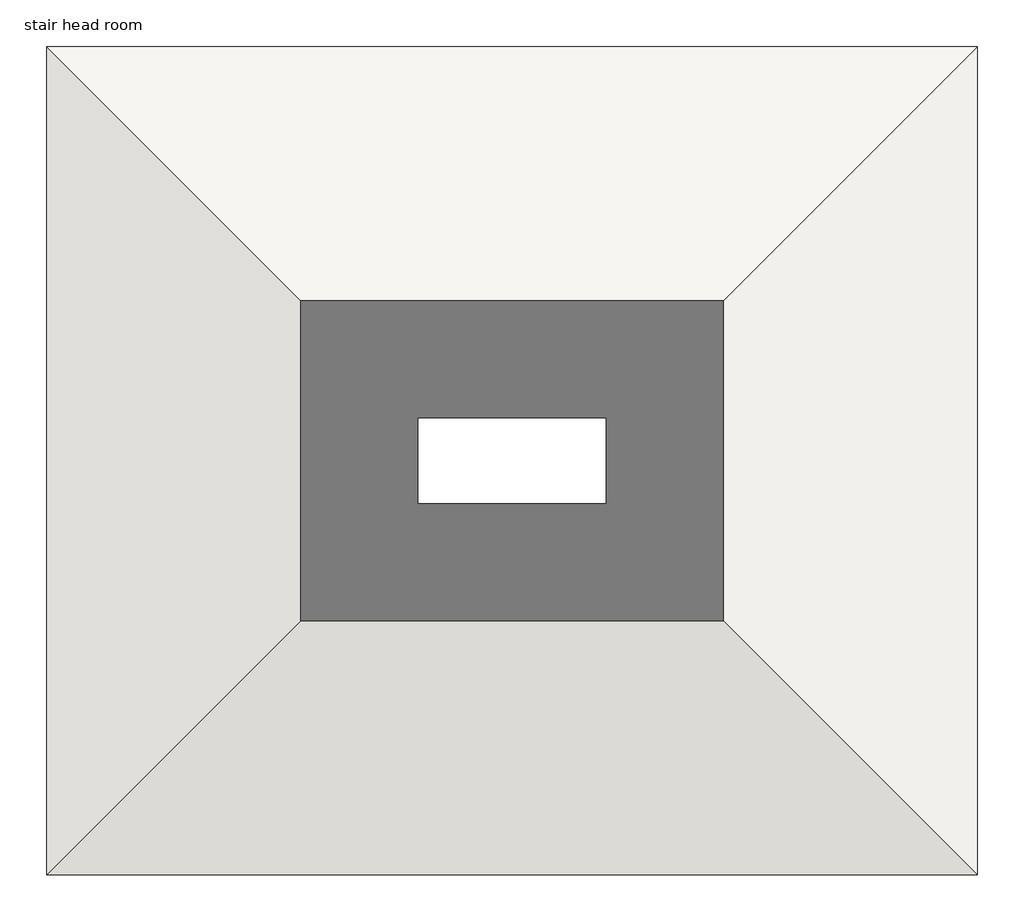
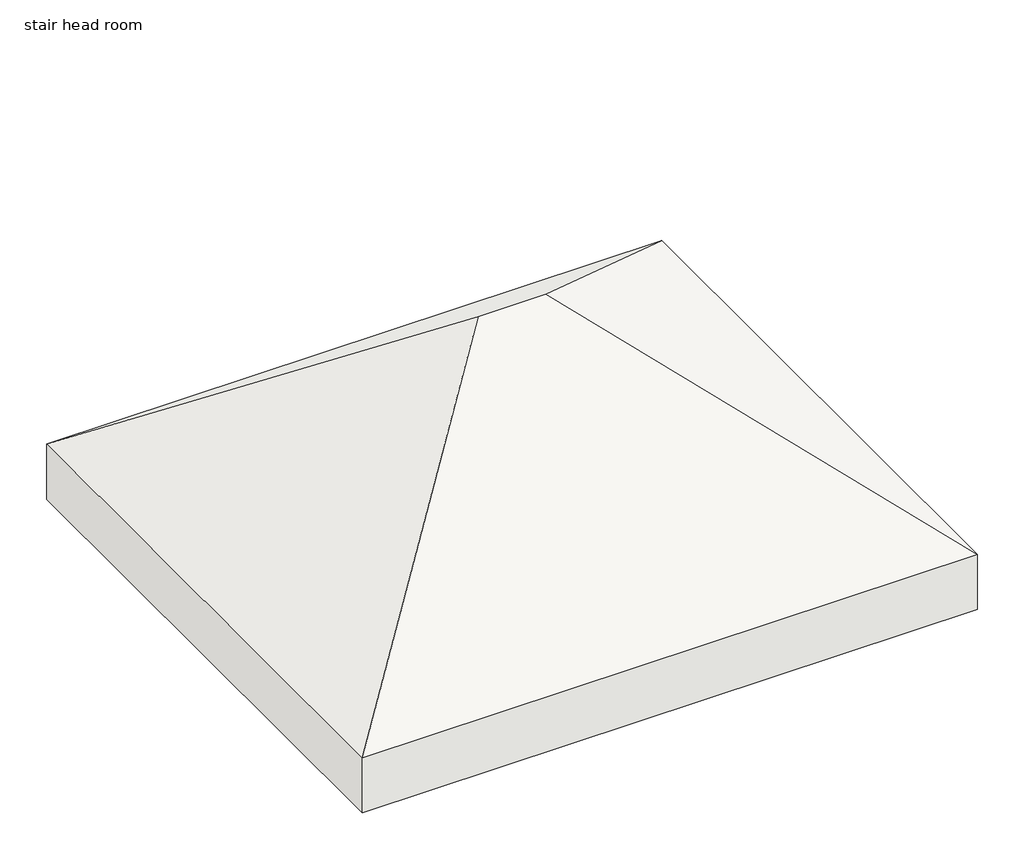
# One storey: 1 roof.
"""IFC4 building model written with IfcOpenShell, lengths in millimetres."""

from ifc_helpers import new_model, si_unit, origin, place, context, project, spatial, faceted_brep, element, save

model = new_model("IFC4")

# Units and contexts
model_context = context("Model", 3, world=origin())
ifc_project = project(units=[si_unit("LENGTHUNIT", "METRE", prefix="MILLI")], contexts=[model_context])

# Site, building, storey
site = spatial("IfcSite", under=ifc_project)
building = spatial("IfcBuilding", under=site)
storey = spatial("IfcBuildingStorey", under=building, Name="stair head room", Elevation=10210.8)

# Roof
placement = place(None, origin())
element("IfcRoof", 1, ObjectType="Generic - 12\"", at=placement, inside=storey, context=model_context, shape_type="Brep", body=[
    faceted_brep([(22524.8636801, 7138.3752787, 10210.8), (20742.1011801, 5355.6127787, 11547.871875), (20300.7761801, 5355.6127787, 11547.871875), (18518.0136801, 7138.3752787, 10210.8), (18518.0136801, 3572.8502787, 10210.8), (22524.8636801, 3572.8502787, 10210.8), (22524.8636801, 7138.3752787, 10591.8), (18518.0136801, 7138.3752787, 10591.8), (20300.7761801, 5355.6127787, 11928.871875), (20742.1011801, 5355.6127787, 11928.871875), (18518.0136801, 3572.8502787, 10591.8), (22524.8636801, 3572.8502787, 10591.8)], [[[0, 1, 2, 3]], [[3, 2, 4]], [[4, 2, 1, 5]], [[1, 0, 5]], [[6, 7, 8, 9]], [[7, 10, 8]], [[10, 11, 9, 8]], [[6, 9, 11]], [[3, 7, 6, 0]], [[4, 10, 7, 3]], [[5, 11, 10, 4]], [[0, 6, 11, 5]]]),
])

save(model, "model.ifc")

# Revit data of these elements
# Type "Generic - 12\""
#   Assembly Code = "B1020"
#   Layers, outside or top first: 1' - 0" no material (function 1)
# Element 1 (IfcRoof, "Generic - 12\"")
#   built-in parameter 1001705 = 39.1367 (stored number, unit not read)
#   built-in parameter 1001710 = 33615
#   Phase Created = New Construction
#   Materials on its faces: "Default Roof"
# Materials
#   "Default Roof": colour RGB 88 101 114, transparency 0, Cost = 0
